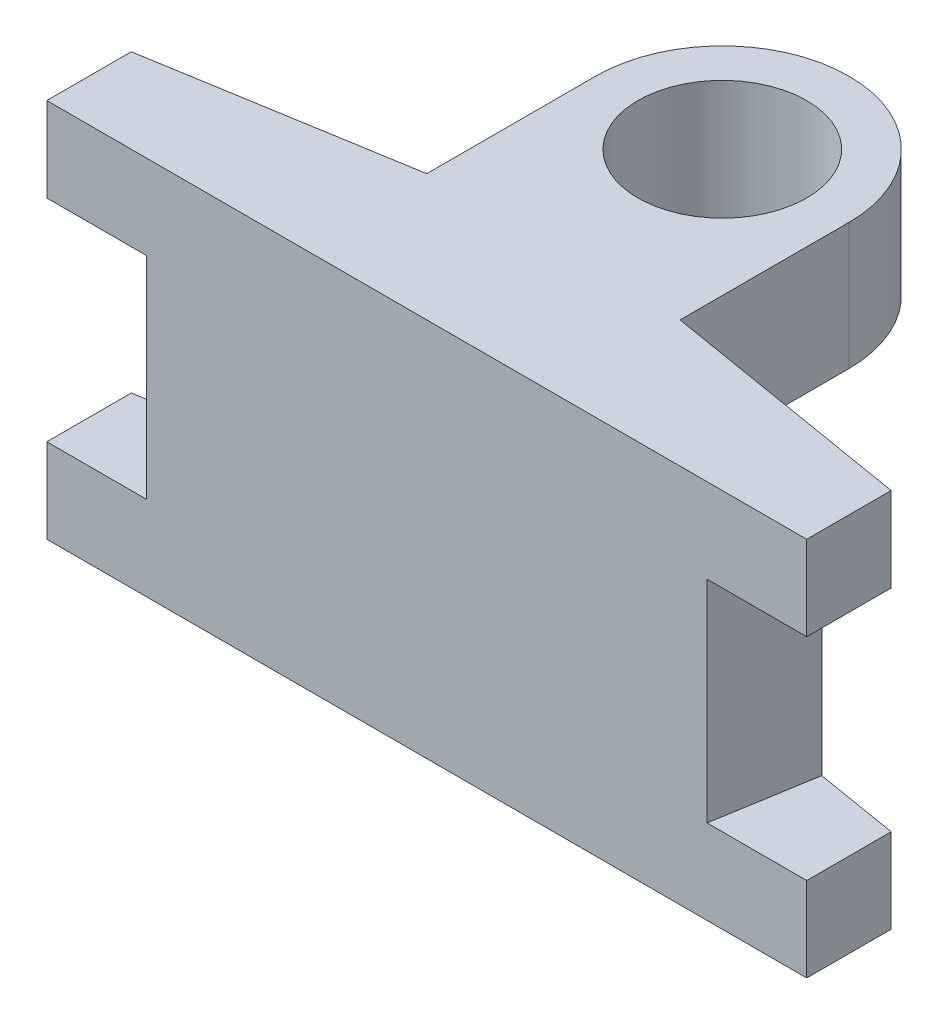
ISO-10303-21;
HEADER;
FILE_DESCRIPTION(('STEP AP214'),'2;1');
FILE_NAME('part.step','',(''),(''),'','','');
FILE_SCHEMA(('AUTOMOTIVE_DESIGN { 1 0 10303 214 1 1 1 1 }'));
ENDSEC;
DATA;
#1=APPLICATION_CONTEXT('core data for automotive mechanical design processes');
#2=APPLICATION_PROTOCOL_DEFINITION('international standard','automotive_design',2000,#1);
#3=PRODUCT_CONTEXT('',#1,'mechanical');
#4=PRODUCT('Part','Part','',(#3));
#5=PRODUCT_RELATED_PRODUCT_CATEGORY('part','',(#4));
#6=PRODUCT_DEFINITION_FORMATION('','',#4);
#7=PRODUCT_DEFINITION_CONTEXT('part definition',#1,'design');
#8=PRODUCT_DEFINITION('design','',#6,#7);
#9=PRODUCT_DEFINITION_SHAPE('','',#8);
#10=(LENGTH_UNIT() NAMED_UNIT(*) SI_UNIT(.MILLI.,.METRE.));
#11=(NAMED_UNIT(*) PLANE_ANGLE_UNIT() SI_UNIT($,.RADIAN.));
#12=(NAMED_UNIT(*) SI_UNIT($,.STERADIAN.) SOLID_ANGLE_UNIT());
#13=UNCERTAINTY_MEASURE_WITH_UNIT(LENGTH_MEASURE(1.E-05),#10,'distance_accuracy_value','');
#14=(GEOMETRIC_REPRESENTATION_CONTEXT(3) GLOBAL_UNCERTAINTY_ASSIGNED_CONTEXT((#13)) GLOBAL_UNIT_ASSIGNED_CONTEXT((#10,
#11,#12)) REPRESENTATION_CONTEXT('',''));
#15=CARTESIAN_POINT('',(0.,0.,0.));
#16=DIRECTION('',(0.,0.,1.));
#17=DIRECTION('',(1.,0.,0.));
#18=AXIS2_PLACEMENT_3D('',#15,#16,#17);
#19=CARTESIAN_POINT('',(0.,0.,20.));
#20=DIRECTION('',(0.,0.,1.));
#21=DIRECTION('',(1.,0.,0.));
#22=AXIS2_PLACEMENT_3D('',#19,#20,#21);
#23=PLANE('',#22);
#24=DIRECTION('',(0.,-1.,0.));
#25=VECTOR('',#24,1.);
#26=CARTESIAN_POINT('',(-33.1921504113325,0.,20.));
#27=LINE('',#26,#25);
#28=CARTESIAN_POINT('',(-33.1921504113325,12.5,20.));
#29=VERTEX_POINT('',#28);
#30=CARTESIAN_POINT('',(-33.1921504113325,-12.5,20.));
#31=VERTEX_POINT('',#30);
#32=EDGE_CURVE('E396',#29,#31,#27,.T.);
#33=ORIENTED_EDGE('',*,*,#32,.T.);
#34=DIRECTION('',(-1.,0.,0.));
#35=VECTOR('',#34,1.);
#36=CARTESIAN_POINT('',(-35.,-12.5,20.));
#37=LINE('',#36,#35);
#38=CARTESIAN_POINT('',(-45.,-12.5,20.));
#39=VERTEX_POINT('',#38);
#40=EDGE_CURVE('E211',#31,#39,#37,.T.);
#41=ORIENTED_EDGE('',*,*,#40,.T.);
#42=DIRECTION('',(0.,-1.,0.));
#43=VECTOR('',#42,1.);
#44=CARTESIAN_POINT('',(-45.,22.5,20.));
#45=LINE('',#44,#43);
#46=CARTESIAN_POINT('',(-45.,-22.5,20.));
#47=VERTEX_POINT('',#46);
#48=EDGE_CURVE('E227',#39,#47,#45,.T.);
#49=ORIENTED_EDGE('',*,*,#48,.T.);
#50=DIRECTION('',(1.,0.,0.));
#51=VECTOR('',#50,1.);
#52=CARTESIAN_POINT('',(15.,-22.5,20.));
#53=LINE('',#52,#51);
#54=CARTESIAN_POINT('',(45.,-22.5,20.));
#55=VERTEX_POINT('',#54);
#56=EDGE_CURVE('E316',#47,#55,#53,.T.);
#57=ORIENTED_EDGE('',*,*,#56,.T.);
#58=DIRECTION('',(0.,-1.,0.));
#59=VECTOR('',#58,1.);
#60=CARTESIAN_POINT('',(45.,22.5,20.));
#61=LINE('',#60,#59);
#62=CARTESIAN_POINT('',(45.,-12.5,20.));
#63=VERTEX_POINT('',#62);
#64=EDGE_CURVE('E268',#63,#55,#61,.T.);
#65=ORIENTED_EDGE('',*,*,#64,.F.);
#66=DIRECTION('',(1.,0.,0.));
#67=VECTOR('',#66,1.);
#68=CARTESIAN_POINT('',(35.,-12.5,20.));
#69=LINE('',#68,#67);
#70=CARTESIAN_POINT('',(33.1921504113325,-12.5,20.));
#71=VERTEX_POINT('',#70);
#72=EDGE_CURVE('E250',#71,#63,#69,.T.);
#73=ORIENTED_EDGE('',*,*,#72,.F.);
#74=DIRECTION('',(0.,-1.,0.));
#75=VECTOR('',#74,1.);
#76=CARTESIAN_POINT('',(33.1921504113325,0.,20.));
#77=LINE('',#76,#75);
#78=CARTESIAN_POINT('',(33.1921504113325,12.5,20.));
#79=VERTEX_POINT('',#78);
#80=EDGE_CURVE('E240',#79,#71,#77,.T.);
#81=ORIENTED_EDGE('',*,*,#80,.F.);
#82=DIRECTION('',(1.,0.,0.));
#83=VECTOR('',#82,1.);
#84=CARTESIAN_POINT('',(35.,12.5,20.));
#85=LINE('',#84,#83);
#86=CARTESIAN_POINT('',(45.,12.5,20.));
#87=VERTEX_POINT('',#86);
#88=EDGE_CURVE('E246',#79,#87,#85,.T.);
#89=ORIENTED_EDGE('',*,*,#88,.T.);
#90=CARTESIAN_POINT('',(45.,22.5,20.));
#91=VERTEX_POINT('',#90);
#92=EDGE_CURVE('E262',#91,#87,#61,.T.);
#93=ORIENTED_EDGE('',*,*,#92,.F.);
#94=DIRECTION('',(-1.,0.,0.));
#95=VECTOR('',#94,1.);
#96=CARTESIAN_POINT('',(15.,22.5,20.));
#97=LINE('',#96,#95);
#98=CARTESIAN_POINT('',(-45.,22.5,20.));
#99=VERTEX_POINT('',#98);
#100=EDGE_CURVE('E317',#91,#99,#97,.T.);
#101=ORIENTED_EDGE('',*,*,#100,.T.);
#102=CARTESIAN_POINT('',(-45.,12.5,20.));
#103=VERTEX_POINT('',#102);
#104=EDGE_CURVE('E225',#99,#103,#45,.T.);
#105=ORIENTED_EDGE('',*,*,#104,.T.);
#106=DIRECTION('',(-1.,0.,0.));
#107=VECTOR('',#106,1.);
#108=CARTESIAN_POINT('',(-35.,12.5,20.));
#109=LINE('',#108,#107);
#110=EDGE_CURVE('E54',#29,#103,#109,.T.);
#111=ORIENTED_EDGE('',*,*,#110,.F.);
#112=EDGE_LOOP('',(#33,#41,#49,#57,#65,#73,#81,#89,#93,#101,#105,#111));
#113=FACE_BOUND('',#112,.T.);
#114=ADVANCED_FACE('F39',(#113),#23,.T.);
#115=CARTESIAN_POINT('',(-45.,22.5,10.));
#116=DIRECTION('',(0.164398987305357,0.,0.986393923832144));
#117=DIRECTION('',(0.986393923832144,0.,-0.164398987305357));
#118=AXIS2_PLACEMENT_3D('',#115,#116,#117);
#119=PLANE('',#118);
#120=DIRECTION('',(0.986393923832144,0.,-0.164398987305358));
#121=VECTOR('',#120,1.);
#122=CARTESIAN_POINT('',(-45.,-12.5,10.));
#123=LINE('',#122,#121);
#124=CARTESIAN_POINT('',(-45.,-12.5,10.));
#125=VERTEX_POINT('',#124);
#126=CARTESIAN_POINT('',(-35.1329031029181,-12.5,8.35548385048635));
#127=VERTEX_POINT('',#126);
#128=EDGE_CURVE('E401',#125,#127,#123,.T.);
#129=ORIENTED_EDGE('',*,*,#128,.T.);
#130=DIRECTION('',(0.,1.,0.));
#131=VECTOR('',#130,1.);
#132=CARTESIAN_POINT('',(-35.1329031029181,-12.5,8.35548385048635));
#133=LINE('',#132,#131);
#134=CARTESIAN_POINT('',(-35.1329031029181,12.5,8.35548385048635));
#135=VERTEX_POINT('',#134);
#136=EDGE_CURVE('E204',#127,#135,#133,.T.);
#137=ORIENTED_EDGE('',*,*,#136,.T.);
#138=DIRECTION('',(-0.986393923832144,0.,0.164398987305357));
#139=VECTOR('',#138,1.);
#140=CARTESIAN_POINT('',(-35.1329031029181,12.5,8.35548385048635));
#141=LINE('',#140,#139);
#142=CARTESIAN_POINT('',(-45.,12.5,10.));
#143=VERTEX_POINT('',#142);
#144=EDGE_CURVE('E197',#135,#143,#141,.T.);
#145=ORIENTED_EDGE('',*,*,#144,.T.);
#146=DIRECTION('',(0.,-1.,0.));
#147=VECTOR('',#146,1.);
#148=CARTESIAN_POINT('',(-45.,22.5,10.));
#149=LINE('',#148,#147);
#150=CARTESIAN_POINT('',(-45.,22.5,10.));
#151=VERTEX_POINT('',#150);
#152=EDGE_CURVE('E203',#151,#143,#149,.T.);
#153=ORIENTED_EDGE('',*,*,#152,.F.);
#154=DIRECTION('',(-0.986393923832144,0.,0.164398987305357));
#155=VECTOR('',#154,1.);
#156=CARTESIAN_POINT('',(-45.,22.5,10.));
#157=LINE('',#156,#155);
#158=CARTESIAN_POINT('',(-15.,22.5,5.));
#159=VERTEX_POINT('',#158);
#160=EDGE_CURVE('E382',#159,#151,#157,.T.);
#161=ORIENTED_EDGE('',*,*,#160,.F.);
#162=DIRECTION('',(0.,-1.,0.));
#163=VECTOR('',#162,1.);
#164=CARTESIAN_POINT('',(-15.,22.5,5.));
#165=LINE('',#164,#163);
#166=CARTESIAN_POINT('',(-15.,-22.5,5.));
#167=VERTEX_POINT('',#166);
#168=EDGE_CURVE('E220',#159,#167,#165,.T.);
#169=ORIENTED_EDGE('',*,*,#168,.T.);
#170=DIRECTION('',(-0.986393923832144,0.,0.164398987305357));
#171=VECTOR('',#170,1.);
#172=CARTESIAN_POINT('',(-45.,-22.5,10.));
#173=LINE('',#172,#171);
#174=CARTESIAN_POINT('',(-45.,-22.5,10.));
#175=VERTEX_POINT('',#174);
#176=EDGE_CURVE('E381',#167,#175,#173,.T.);
#177=ORIENTED_EDGE('',*,*,#176,.T.);
#178=EDGE_CURVE('E217',#125,#175,#149,.T.);
#179=ORIENTED_EDGE('',*,*,#178,.F.);
#180=EDGE_LOOP('',(#129,#137,#145,#153,#161,#169,#177,#179));
#181=FACE_BOUND('',#180,.T.);
#182=ADVANCED_FACE('F200',(#181),#119,.F.);
#183=CARTESIAN_POINT('',(-45.,22.5,20.));
#184=DIRECTION('',(1.,0.,0.));
#185=DIRECTION('',(0.,0.,-1.));
#186=AXIS2_PLACEMENT_3D('',#183,#184,#185);
#187=PLANE('',#186);
#188=DIRECTION('',(0.,0.,-1.));
#189=VECTOR('',#188,1.);
#190=CARTESIAN_POINT('',(-45.,-12.5,20.));
#191=LINE('',#190,#189);
#192=EDGE_CURVE('E215',#39,#125,#191,.T.);
#193=ORIENTED_EDGE('',*,*,#192,.T.);
#194=ORIENTED_EDGE('',*,*,#178,.T.);
#195=DIRECTION('',(0.,0.,1.));
#196=VECTOR('',#195,1.);
#197=CARTESIAN_POINT('',(-45.,-22.5,20.));
#198=LINE('',#197,#196);
#199=EDGE_CURVE('E389',#175,#47,#198,.T.);
#200=ORIENTED_EDGE('',*,*,#199,.T.);
#201=ORIENTED_EDGE('',*,*,#48,.F.);
#202=EDGE_LOOP('',(#193,#194,#200,#201));
#203=FACE_BOUND('',#202,.T.);
#204=ADVANCED_FACE('F411',(#203),#187,.F.);
#205=DIRECTION('',(0.,0.,1.));
#206=VECTOR('',#205,1.);
#207=CARTESIAN_POINT('',(-45.,12.5,20.));
#208=LINE('',#207,#206);
#209=EDGE_CURVE('E206',#143,#103,#208,.T.);
#210=ORIENTED_EDGE('',*,*,#209,.T.);
#211=ORIENTED_EDGE('',*,*,#104,.F.);
#212=DIRECTION('',(0.,0.,1.));
#213=VECTOR('',#212,1.);
#214=CARTESIAN_POINT('',(-45.,22.5,20.));
#215=LINE('',#214,#213);
#216=EDGE_CURVE('E216',#151,#99,#215,.T.);
#217=ORIENTED_EDGE('',*,*,#216,.F.);
#218=ORIENTED_EDGE('',*,*,#152,.T.);
#219=EDGE_LOOP('',(#210,#211,#217,#218));
#220=FACE_BOUND('',#219,.T.);
#221=ADVANCED_FACE('F212',(#220),#187,.F.);
#222=CARTESIAN_POINT('',(-15.,-22.5,20.));
#223=DIRECTION('',(1.,0.,0.));
#224=DIRECTION('',(0.,0.,-1.));
#225=AXIS2_PLACEMENT_3D('',#222,#223,#224);
#226=PLANE('',#225);
#227=ORIENTED_EDGE('',*,*,#168,.F.);
#228=DIRECTION('',(0.,0.,-1.));
#229=VECTOR('',#228,1.);
#230=CARTESIAN_POINT('',(-15.,22.5,20.));
#231=LINE('',#230,#229);
#232=CARTESIAN_POINT('',(-15.,22.5,-15.));
#233=VERTEX_POINT('',#232);
#234=EDGE_CURVE('E325',#159,#233,#231,.T.);
#235=ORIENTED_EDGE('',*,*,#234,.T.);
#236=DIRECTION('',(0.,1.,0.));
#237=VECTOR('',#236,1.);
#238=CARTESIAN_POINT('',(-15.,7.50000000000001,-15.));
#239=LINE('',#238,#237);
#240=CARTESIAN_POINT('',(-15.,7.50000000000001,-15.));
#241=VERTEX_POINT('',#240);
#242=EDGE_CURVE('E345',#233,#241,#239,.F.);
#243=ORIENTED_EDGE('',*,*,#242,.T.);
#244=DIRECTION('',(0.,0.,1.));
#245=VECTOR('',#244,1.);
#246=CARTESIAN_POINT('',(-15.,7.50000000000001,-30.));
#247=LINE('',#246,#245);
#248=CARTESIAN_POINT('',(-15.,7.50000000000001,0.));
#249=VERTEX_POINT('',#248);
#250=EDGE_CURVE('E283',#241,#249,#247,.T.);
#251=ORIENTED_EDGE('',*,*,#250,.T.);
#252=DIRECTION('',(0.,-1.,0.));
#253=VECTOR('',#252,1.);
#254=CARTESIAN_POINT('',(-15.,-22.5,0.));
#255=LINE('',#254,#253);
#256=CARTESIAN_POINT('',(-15.,-22.5,0.));
#257=VERTEX_POINT('',#256);
#258=EDGE_CURVE('E306',#249,#257,#255,.T.);
#259=ORIENTED_EDGE('',*,*,#258,.T.);
#260=DIRECTION('',(0.,0.,-1.));
#261=VECTOR('',#260,1.);
#262=CARTESIAN_POINT('',(-15.,-22.5,20.));
#263=LINE('',#262,#261);
#264=EDGE_CURVE('E337',#167,#257,#263,.T.);
#265=ORIENTED_EDGE('',*,*,#264,.F.);
#266=EDGE_LOOP('',(#227,#235,#243,#251,#259,#265));
#267=FACE_BOUND('',#266,.T.);
#268=ADVANCED_FACE('F380',(#267),#226,.F.);
#269=CARTESIAN_POINT('',(45.,22.5,20.));
#270=DIRECTION('',(1.,0.,0.));
#271=DIRECTION('',(0.,0.,-1.));
#272=AXIS2_PLACEMENT_3D('',#269,#270,#271);
#273=PLANE('',#272);
#274=DIRECTION('',(0.,0.,-1.));
#275=VECTOR('',#274,1.);
#276=CARTESIAN_POINT('',(45.,-12.5,20.));
#277=LINE('',#276,#275);
#278=CARTESIAN_POINT('',(45.,-12.5,10.));
#279=VERTEX_POINT('',#278);
#280=EDGE_CURVE('E242',#63,#279,#277,.T.);
#281=ORIENTED_EDGE('',*,*,#280,.F.);
#282=ORIENTED_EDGE('',*,*,#64,.T.);
#283=DIRECTION('',(0.,0.,1.));
#284=VECTOR('',#283,1.);
#285=CARTESIAN_POINT('',(45.,-22.5,20.));
#286=LINE('',#285,#284);
#287=CARTESIAN_POINT('',(45.,-22.5,10.));
#288=VERTEX_POINT('',#287);
#289=EDGE_CURVE('E258',#288,#55,#286,.T.);
#290=ORIENTED_EDGE('',*,*,#289,.F.);
#291=DIRECTION('',(0.,-1.,0.));
#292=VECTOR('',#291,1.);
#293=CARTESIAN_POINT('',(45.,22.5,10.));
#294=LINE('',#293,#292);
#295=EDGE_CURVE('E275',#279,#288,#294,.T.);
#296=ORIENTED_EDGE('',*,*,#295,.F.);
#297=EDGE_LOOP('',(#281,#282,#290,#296));
#298=FACE_BOUND('',#297,.T.);
#299=ADVANCED_FACE('F419',(#298),#273,.T.);
#300=CARTESIAN_POINT('',(0.,0.,0.));
#301=DIRECTION('',(0.,0.,1.));
#302=DIRECTION('',(1.,0.,0.));
#303=AXIS2_PLACEMENT_3D('',#300,#301,#302);
#304=PLANE('',#303);
#305=DIRECTION('',(-1.,0.,0.));
#306=VECTOR('',#305,1.);
#307=CARTESIAN_POINT('',(15.,7.50000000000001,0.));
#308=LINE('',#307,#306);
#309=CARTESIAN_POINT('',(15.,7.5,0.));
#310=VERTEX_POINT('',#309);
#311=EDGE_CURVE('E278',#310,#249,#308,.T.);
#312=ORIENTED_EDGE('',*,*,#311,.F.);
#313=DIRECTION('',(0.,1.,0.));
#314=VECTOR('',#313,1.);
#315=CARTESIAN_POINT('',(15.,-22.5,0.));
#316=LINE('',#315,#314);
#317=CARTESIAN_POINT('',(15.,-22.5,0.));
#318=VERTEX_POINT('',#317);
#319=EDGE_CURVE('E319',#318,#310,#316,.T.);
#320=ORIENTED_EDGE('',*,*,#319,.F.);
#321=DIRECTION('',(1.,0.,0.));
#322=VECTOR('',#321,1.);
#323=CARTESIAN_POINT('',(15.,-22.5,0.));
#324=LINE('',#323,#322);
#325=CARTESIAN_POINT('',(9.99999999999999,-22.5,0.));
#326=VERTEX_POINT('',#325);
#327=EDGE_CURVE('E324',#326,#318,#324,.T.);
#328=ORIENTED_EDGE('',*,*,#327,.F.);
#329=DIRECTION('',(0.,-1.,0.));
#330=VECTOR('',#329,1.);
#331=CARTESIAN_POINT('',(10.,-7.5,0.));
#332=LINE('',#331,#330);
#333=CARTESIAN_POINT('',(10.,-7.5,0.));
#334=VERTEX_POINT('',#333);
#335=EDGE_CURVE('E301',#334,#326,#332,.T.);
#336=ORIENTED_EDGE('',*,*,#335,.F.);
#337=CARTESIAN_POINT('',(0.,-7.49999999999999,0.));
#338=DIRECTION('',(0.,0.,-1.));
#339=DIRECTION('',(-1.,0.,0.));
#340=AXIS2_PLACEMENT_3D('',#337,#338,#339);
#341=CIRCLE('',#340,10.);
#342=CARTESIAN_POINT('',(-10.,-7.49999999999999,0.));
#343=VERTEX_POINT('',#342);
#344=EDGE_CURVE('E286',#343,#334,#341,.T.);
#345=ORIENTED_EDGE('',*,*,#344,.F.);
#346=DIRECTION('',(0.,1.,0.));
#347=VECTOR('',#346,1.);
#348=CARTESIAN_POINT('',(-10.,-22.5,0.));
#349=LINE('',#348,#347);
#350=CARTESIAN_POINT('',(-10.,-22.5,0.));
#351=VERTEX_POINT('',#350);
#352=EDGE_CURVE('E295',#351,#343,#349,.T.);
#353=ORIENTED_EDGE('',*,*,#352,.F.);
#354=EDGE_CURVE('E326',#257,#351,#324,.T.);
#355=ORIENTED_EDGE('',*,*,#354,.F.);
#356=ORIENTED_EDGE('',*,*,#258,.F.);
#357=EDGE_LOOP('',(#312,#320,#328,#336,#345,#353,#355,#356));
#358=FACE_BOUND('',#357,.T.);
#359=ADVANCED_FACE('F367',(#358),#304,.F.);
#360=CARTESIAN_POINT('',(15.,-22.5,20.));
#361=DIRECTION('',(0.,1.,0.));
#362=DIRECTION('',(0.,0.,1.));
#363=AXIS2_PLACEMENT_3D('',#360,#361,#362);
#364=PLANE('',#363);
#365=ORIENTED_EDGE('',*,*,#354,.T.);
#366=DIRECTION('',(0.,0.,-1.));
#367=VECTOR('',#366,1.);
#368=CARTESIAN_POINT('',(-10.,-22.5,8.));
#369=LINE('',#368,#367);
#370=CARTESIAN_POINT('',(-10.,-22.5,8.));
#371=VERTEX_POINT('',#370);
#372=EDGE_CURVE('E310',#371,#351,#369,.T.);
#373=ORIENTED_EDGE('',*,*,#372,.F.);
#374=DIRECTION('',(-1.,0.,0.));
#375=VECTOR('',#374,1.);
#376=CARTESIAN_POINT('',(9.99999999999999,-22.5,8.));
#377=LINE('',#376,#375);
#378=CARTESIAN_POINT('',(9.99999999999999,-22.5,8.));
#379=VERTEX_POINT('',#378);
#380=EDGE_CURVE('E293',#379,#371,#377,.T.);
#381=ORIENTED_EDGE('',*,*,#380,.F.);
#382=DIRECTION('',(0.,0.,-1.));
#383=VECTOR('',#382,1.);
#384=CARTESIAN_POINT('',(9.99999999999999,-22.5,8.));
#385=LINE('',#384,#383);
#386=EDGE_CURVE('E313',#379,#326,#385,.T.);
#387=ORIENTED_EDGE('',*,*,#386,.T.);
#388=ORIENTED_EDGE('',*,*,#327,.T.);
#389=DIRECTION('',(0.,0.,-1.));
#390=VECTOR('',#389,1.);
#391=CARTESIAN_POINT('',(15.,-22.5,20.));
#392=LINE('',#391,#390);
#393=CARTESIAN_POINT('',(15.,-22.5,5.));
#394=VERTEX_POINT('',#393);
#395=EDGE_CURVE('E331',#394,#318,#392,.T.);
#396=ORIENTED_EDGE('',*,*,#395,.F.);
#397=DIRECTION('',(0.986393923832144,0.,0.164398987305357));
#398=VECTOR('',#397,1.);
#399=CARTESIAN_POINT('',(45.,-22.5,10.));
#400=LINE('',#399,#398);
#401=EDGE_CURVE('E247',#394,#288,#400,.T.);
#402=ORIENTED_EDGE('',*,*,#401,.T.);
#403=ORIENTED_EDGE('',*,*,#289,.T.);
#404=ORIENTED_EDGE('',*,*,#56,.F.);
#405=ORIENTED_EDGE('',*,*,#199,.F.);
#406=ORIENTED_EDGE('',*,*,#176,.F.);
#407=ORIENTED_EDGE('',*,*,#264,.T.);
#408=EDGE_LOOP('',(#365,#373,#381,#387,#388,#396,#402,#403,#404,#405,#406,#407));
#409=FACE_BOUND('',#408,.T.);
#410=ADVANCED_FACE('F384',(#409),#364,.F.);
#411=CARTESIAN_POINT('',(15.,-22.5,20.));
#412=DIRECTION('',(-1.,0.,0.));
#413=DIRECTION('',(0.,0.,1.));
#414=AXIS2_PLACEMENT_3D('',#411,#412,#413);
#415=PLANE('',#414);
#416=DIRECTION('',(0.,0.,-1.));
#417=VECTOR('',#416,1.);
#418=CARTESIAN_POINT('',(15.,22.5,20.));
#419=LINE('',#418,#417);
#420=CARTESIAN_POINT('',(15.,22.5,5.));
#421=VERTEX_POINT('',#420);
#422=CARTESIAN_POINT('',(15.,22.5,-15.));
#423=VERTEX_POINT('',#422);
#424=EDGE_CURVE('E335',#421,#423,#419,.T.);
#425=ORIENTED_EDGE('',*,*,#424,.F.);
#426=DIRECTION('',(0.,-1.,0.));
#427=VECTOR('',#426,1.);
#428=CARTESIAN_POINT('',(15.,22.5,5.));
#429=LINE('',#428,#427);
#430=EDGE_CURVE('E259',#421,#394,#429,.T.);
#431=ORIENTED_EDGE('',*,*,#430,.T.);
#432=ORIENTED_EDGE('',*,*,#395,.T.);
#433=ORIENTED_EDGE('',*,*,#319,.T.);
#434=DIRECTION('',(0.,0.,1.));
#435=VECTOR('',#434,1.);
#436=CARTESIAN_POINT('',(15.,7.50000000000001,-30.));
#437=LINE('',#436,#435);
#438=CARTESIAN_POINT('',(15.,7.50000000000001,-15.));
#439=VERTEX_POINT('',#438);
#440=EDGE_CURVE('E281',#439,#310,#437,.T.);
#441=ORIENTED_EDGE('',*,*,#440,.F.);
#442=DIRECTION('',(0.,-1.,0.));
#443=VECTOR('',#442,1.);
#444=CARTESIAN_POINT('',(15.,22.5,-15.));
#445=LINE('',#444,#443);
#446=EDGE_CURVE('E11',#439,#423,#445,.F.);
#447=ORIENTED_EDGE('',*,*,#446,.T.);
#448=EDGE_LOOP('',(#425,#431,#432,#433,#441,#447));
#449=FACE_BOUND('',#448,.T.);
#450=ADVANCED_FACE('F364',(#449),#415,.F.);
#451=CARTESIAN_POINT('',(15.,22.5,20.));
#452=DIRECTION('',(0.,-1.,0.));
#453=DIRECTION('',(0.,0.,-1.));
#454=AXIS2_PLACEMENT_3D('',#451,#452,#453);
#455=PLANE('',#454);
#456=CARTESIAN_POINT('',(0.,22.5,-15.));
#457=DIRECTION('',(0.,-1.,0.));
#458=DIRECTION('',(0.,0.,-1.));
#459=AXIS2_PLACEMENT_3D('',#456,#457,#458);
#460=CIRCLE('',#459,10.);
#461=CARTESIAN_POINT('',(0.,22.5,-25.));
#462=VERTEX_POINT('',#461);
#463=EDGE_CURVE('E280',#462,#462,#460,.T.);
#464=ORIENTED_EDGE('',*,*,#463,.T.);
#465=EDGE_LOOP('',(#464));
#466=FACE_BOUND('',#465,.T.);
#467=CARTESIAN_POINT('',(0.,22.5,-15.));
#468=DIRECTION('',(0.,-1.,0.));
#469=DIRECTION('',(0.,0.,-1.));
#470=AXIS2_PLACEMENT_3D('',#467,#468,#469);
#471=CIRCLE('',#470,15.);
#472=CARTESIAN_POINT('',(0.,22.5,-30.));
#473=VERTEX_POINT('',#472);
#474=EDGE_CURVE('E338',#423,#473,#471,.F.);
#475=ORIENTED_EDGE('',*,*,#474,.T.);
#476=CARTESIAN_POINT('',(0.,22.5,-15.));
#477=DIRECTION('',(0.,-1.,0.));
#478=DIRECTION('',(0.,0.,-1.));
#479=AXIS2_PLACEMENT_3D('',#476,#477,#478);
#480=CIRCLE('',#479,15.);
#481=EDGE_CURVE('E336',#473,#233,#480,.F.);
#482=ORIENTED_EDGE('',*,*,#481,.T.);
#483=ORIENTED_EDGE('',*,*,#234,.F.);
#484=ORIENTED_EDGE('',*,*,#160,.T.);
#485=ORIENTED_EDGE('',*,*,#216,.T.);
#486=ORIENTED_EDGE('',*,*,#100,.F.);
#487=DIRECTION('',(0.,0.,1.));
#488=VECTOR('',#487,1.);
#489=CARTESIAN_POINT('',(45.,22.5,20.));
#490=LINE('',#489,#488);
#491=CARTESIAN_POINT('',(45.,22.5,10.));
#492=VERTEX_POINT('',#491);
#493=EDGE_CURVE('E254',#492,#91,#490,.T.);
#494=ORIENTED_EDGE('',*,*,#493,.F.);
#495=DIRECTION('',(0.986393923832144,0.,0.164398987305357));
#496=VECTOR('',#495,1.);
#497=CARTESIAN_POINT('',(45.,22.5,10.));
#498=LINE('',#497,#496);
#499=EDGE_CURVE('E252',#421,#492,#498,.T.);
#500=ORIENTED_EDGE('',*,*,#499,.F.);
#501=ORIENTED_EDGE('',*,*,#424,.T.);
#502=EDGE_LOOP('',(#475,#482,#483,#484,#485,#486,#494,#500,#501));
#503=FACE_BOUND('',#502,.T.);
#504=ADVANCED_FACE('F357',(#466,#503),#455,.F.);
#505=CARTESIAN_POINT('',(0.,-7.49999999999999,8.));
#506=DIRECTION('',(0.,0.,-1.));
#507=DIRECTION('',(-1.,0.,0.));
#508=AXIS2_PLACEMENT_3D('',#505,#506,#507);
#509=CYLINDRICAL_SURFACE('',#508,10.);
#510=ORIENTED_EDGE('',*,*,#344,.T.);
#511=DIRECTION('',(0.,0.,-1.));
#512=VECTOR('',#511,1.);
#513=CARTESIAN_POINT('',(10.,-7.5,8.));
#514=LINE('',#513,#512);
#515=CARTESIAN_POINT('',(10.,-7.5,8.));
#516=VERTEX_POINT('',#515);
#517=EDGE_CURVE('E296',#516,#334,#514,.T.);
#518=ORIENTED_EDGE('',*,*,#517,.F.);
#519=CARTESIAN_POINT('',(0.,-7.49999999999999,8.));
#520=DIRECTION('',(0.,0.,-1.));
#521=DIRECTION('',(-1.,0.,0.));
#522=AXIS2_PLACEMENT_3D('',#519,#520,#521);
#523=CIRCLE('',#522,10.);
#524=CARTESIAN_POINT('',(-10.,-7.49999999999999,8.));
#525=VERTEX_POINT('',#524);
#526=EDGE_CURVE('E290',#525,#516,#523,.T.);
#527=ORIENTED_EDGE('',*,*,#526,.F.);
#528=DIRECTION('',(0.,0.,-1.));
#529=VECTOR('',#528,1.);
#530=CARTESIAN_POINT('',(-10.,-7.49999999999999,8.));
#531=LINE('',#530,#529);
#532=EDGE_CURVE('E308',#525,#343,#531,.T.);
#533=ORIENTED_EDGE('',*,*,#532,.T.);
#534=EDGE_LOOP('',(#510,#518,#527,#533));
#535=FACE_BOUND('',#534,.T.);
#536=ADVANCED_FACE('F457',(#535),#509,.F.);
#537=CARTESIAN_POINT('',(-10.,-22.5,8.));
#538=DIRECTION('',(-1.,0.,0.));
#539=DIRECTION('',(0.,-1.,0.));
#540=AXIS2_PLACEMENT_3D('',#537,#538,#539);
#541=PLANE('',#540);
#542=ORIENTED_EDGE('',*,*,#352,.T.);
#543=ORIENTED_EDGE('',*,*,#532,.F.);
#544=DIRECTION('',(0.,1.,0.));
#545=VECTOR('',#544,1.);
#546=CARTESIAN_POINT('',(-10.,-22.5,8.));
#547=LINE('',#546,#545);
#548=EDGE_CURVE('E300',#371,#525,#547,.T.);
#549=ORIENTED_EDGE('',*,*,#548,.F.);
#550=ORIENTED_EDGE('',*,*,#372,.T.);
#551=EDGE_LOOP('',(#542,#543,#549,#550));
#552=FACE_BOUND('',#551,.T.);
#553=ADVANCED_FACE('F491',(#552),#541,.F.);
#554=CARTESIAN_POINT('',(10.,-7.5,8.));
#555=DIRECTION('',(1.,0.,0.));
#556=DIRECTION('',(0.,1.,0.));
#557=AXIS2_PLACEMENT_3D('',#554,#555,#556);
#558=PLANE('',#557);
#559=ORIENTED_EDGE('',*,*,#335,.T.);
#560=ORIENTED_EDGE('',*,*,#386,.F.);
#561=DIRECTION('',(0.,-1.,0.));
#562=VECTOR('',#561,1.);
#563=CARTESIAN_POINT('',(10.,-7.5,8.));
#564=LINE('',#563,#562);
#565=EDGE_CURVE('E292',#516,#379,#564,.T.);
#566=ORIENTED_EDGE('',*,*,#565,.F.);
#567=ORIENTED_EDGE('',*,*,#517,.T.);
#568=EDGE_LOOP('',(#559,#560,#566,#567));
#569=FACE_BOUND('',#568,.T.);
#570=ADVANCED_FACE('F484',(#569),#558,.F.);
#571=CARTESIAN_POINT('',(0.,-7.49999999999999,8.));
#572=DIRECTION('',(0.,0.,-1.));
#573=DIRECTION('',(-1.,0.,0.));
#574=AXIS2_PLACEMENT_3D('',#571,#572,#573);
#575=PLANE('',#574);
#576=ORIENTED_EDGE('',*,*,#526,.T.);
#577=ORIENTED_EDGE('',*,*,#565,.T.);
#578=ORIENTED_EDGE('',*,*,#380,.T.);
#579=ORIENTED_EDGE('',*,*,#548,.T.);
#580=EDGE_LOOP('',(#576,#577,#578,#579));
#581=FACE_BOUND('',#580,.T.);
#582=ADVANCED_FACE('F479',(#581),#575,.T.);
#583=CARTESIAN_POINT('',(15.,7.50000000000001,-30.));
#584=DIRECTION('',(0.,1.,0.));
#585=DIRECTION('',(0.,0.,1.));
#586=AXIS2_PLACEMENT_3D('',#583,#584,#585);
#587=PLANE('',#586);
#588=CARTESIAN_POINT('',(0.,7.50000000000001,-15.));
#589=DIRECTION('',(0.,-1.,0.));
#590=DIRECTION('',(0.,0.,-1.));
#591=AXIS2_PLACEMENT_3D('',#588,#589,#590);
#592=CIRCLE('',#591,10.);
#593=CARTESIAN_POINT('',(0.,7.50000000000001,-25.));
#594=VERTEX_POINT('',#593);
#595=EDGE_CURVE('E270',#594,#594,#592,.T.);
#596=ORIENTED_EDGE('',*,*,#595,.F.);
#597=EDGE_LOOP('',(#596));
#598=FACE_BOUND('',#597,.T.);
#599=ORIENTED_EDGE('',*,*,#250,.F.);
#600=CARTESIAN_POINT('',(0.,7.50000000000001,-15.));
#601=DIRECTION('',(0.,1.,0.));
#602=DIRECTION('',(0.,0.,1.));
#603=AXIS2_PLACEMENT_3D('',#600,#601,#602);
#604=CIRCLE('',#603,15.);
#605=CARTESIAN_POINT('',(0.,7.50000000000001,-30.));
#606=VERTEX_POINT('',#605);
#607=EDGE_CURVE('E48',#241,#606,#604,.F.);
#608=ORIENTED_EDGE('',*,*,#607,.T.);
#609=CARTESIAN_POINT('',(0.,7.50000000000001,-15.));
#610=DIRECTION('',(0.,1.,0.));
#611=DIRECTION('',(0.,0.,1.));
#612=AXIS2_PLACEMENT_3D('',#609,#610,#611);
#613=CIRCLE('',#612,15.);
#614=EDGE_CURVE('E63',#606,#439,#613,.F.);
#615=ORIENTED_EDGE('',*,*,#614,.T.);
#616=ORIENTED_EDGE('',*,*,#440,.T.);
#617=ORIENTED_EDGE('',*,*,#311,.T.);
#618=EDGE_LOOP('',(#599,#608,#615,#616,#617));
#619=FACE_BOUND('',#618,.T.);
#620=ADVANCED_FACE('F346',(#598,#619),#587,.F.);
#621=CARTESIAN_POINT('',(0.,0.,-15.));
#622=DIRECTION('',(0.,1.,0.));
#623=DIRECTION('',(0.,0.,1.));
#624=AXIS2_PLACEMENT_3D('',#621,#622,#623);
#625=CYLINDRICAL_SURFACE('',#624,15.);
#626=ORIENTED_EDGE('',*,*,#446,.F.);
#627=ORIENTED_EDGE('',*,*,#614,.F.);
#628=DIRECTION('',(0.,-1.,0.));
#629=VECTOR('',#628,1.);
#630=CARTESIAN_POINT('',(0.,7.50000000000001,-30.));
#631=LINE('',#630,#629);
#632=EDGE_CURVE('E43',#473,#606,#631,.T.);
#633=ORIENTED_EDGE('',*,*,#632,.F.);
#634=ORIENTED_EDGE('',*,*,#474,.F.);
#635=EDGE_LOOP('',(#626,#627,#633,#634));
#636=FACE_BOUND('',#635,.T.);
#637=ADVANCED_FACE('F41',(#636),#625,.T.);
#638=CARTESIAN_POINT('',(0.,0.,-15.));
#639=DIRECTION('',(0.,-1.,0.));
#640=DIRECTION('',(0.,0.,-1.));
#641=AXIS2_PLACEMENT_3D('',#638,#639,#640);
#642=CYLINDRICAL_SURFACE('',#641,15.);
#643=ORIENTED_EDGE('',*,*,#607,.F.);
#644=ORIENTED_EDGE('',*,*,#242,.F.);
#645=ORIENTED_EDGE('',*,*,#481,.F.);
#646=ORIENTED_EDGE('',*,*,#632,.T.);
#647=EDGE_LOOP('',(#643,#644,#645,#646));
#648=FACE_BOUND('',#647,.T.);
#649=ADVANCED_FACE('F356',(#648),#642,.T.);
#650=CARTESIAN_POINT('',(0.,37.5,-15.));
#651=DIRECTION('',(0.,-1.,0.));
#652=DIRECTION('',(0.,0.,-1.));
#653=AXIS2_PLACEMENT_3D('',#650,#651,#652);
#654=CYLINDRICAL_SURFACE('',#653,10.);
#655=ORIENTED_EDGE('',*,*,#595,.T.);
#656=EDGE_LOOP('',(#655));
#657=FACE_BOUND('',#656,.T.);
#658=ORIENTED_EDGE('',*,*,#463,.F.);
#659=EDGE_LOOP('',(#658));
#660=FACE_BOUND('',#659,.T.);
#661=ADVANCED_FACE('F468',(#657,#660),#654,.F.);
#662=DIRECTION('',(0.,0.,1.));
#663=VECTOR('',#662,1.);
#664=CARTESIAN_POINT('',(45.,12.5,20.));
#665=LINE('',#664,#663);
#666=CARTESIAN_POINT('',(45.,12.5,10.));
#667=VERTEX_POINT('',#666);
#668=EDGE_CURVE('E244',#667,#87,#665,.T.);
#669=ORIENTED_EDGE('',*,*,#668,.F.);
#670=EDGE_CURVE('E267',#492,#667,#294,.T.);
#671=ORIENTED_EDGE('',*,*,#670,.F.);
#672=ORIENTED_EDGE('',*,*,#493,.T.);
#673=ORIENTED_EDGE('',*,*,#92,.T.);
#674=EDGE_LOOP('',(#669,#671,#672,#673));
#675=FACE_BOUND('',#674,.T.);
#676=ADVANCED_FACE('F436',(#675),#273,.T.);
#677=CARTESIAN_POINT('',(45.,22.5,10.));
#678=DIRECTION('',(0.164398987305357,0.,-0.986393923832144));
#679=DIRECTION('',(-0.986393923832144,0.,-0.164398987305357));
#680=AXIS2_PLACEMENT_3D('',#677,#678,#679);
#681=PLANE('',#680);
#682=DIRECTION('',(0.986393923832144,0.,0.164398987305357));
#683=VECTOR('',#682,1.);
#684=CARTESIAN_POINT('',(35.1329031029181,12.5,8.35548385048635));
#685=LINE('',#684,#683);
#686=CARTESIAN_POINT('',(35.1329031029181,12.5,8.35548385048635));
#687=VERTEX_POINT('',#686);
#688=EDGE_CURVE('E231',#687,#667,#685,.T.);
#689=ORIENTED_EDGE('',*,*,#688,.F.);
#690=DIRECTION('',(0.,1.,0.));
#691=VECTOR('',#690,1.);
#692=CARTESIAN_POINT('',(35.1329031029181,-12.5,8.35548385048635));
#693=LINE('',#692,#691);
#694=CARTESIAN_POINT('',(35.1329031029181,-12.5,8.35548385048635));
#695=VERTEX_POINT('',#694);
#696=EDGE_CURVE('E229',#695,#687,#693,.T.);
#697=ORIENTED_EDGE('',*,*,#696,.F.);
#698=DIRECTION('',(-0.986393923832144,0.,-0.164398987305358));
#699=VECTOR('',#698,1.);
#700=CARTESIAN_POINT('',(45.,-12.5,10.));
#701=LINE('',#700,#699);
#702=EDGE_CURVE('E219',#279,#695,#701,.T.);
#703=ORIENTED_EDGE('',*,*,#702,.F.);
#704=ORIENTED_EDGE('',*,*,#295,.T.);
#705=ORIENTED_EDGE('',*,*,#401,.F.);
#706=ORIENTED_EDGE('',*,*,#430,.F.);
#707=ORIENTED_EDGE('',*,*,#499,.T.);
#708=ORIENTED_EDGE('',*,*,#670,.T.);
#709=EDGE_LOOP('',(#689,#697,#703,#704,#705,#706,#707,#708));
#710=FACE_BOUND('',#709,.T.);
#711=ADVANCED_FACE('F431',(#710),#681,.T.);
#712=CARTESIAN_POINT('',(35.,-12.5,20.));
#713=DIRECTION('',(0.,-1.,0.));
#714=DIRECTION('',(0.,0.,-1.));
#715=AXIS2_PLACEMENT_3D('',#712,#713,#714);
#716=PLANE('',#715);
#717=ORIENTED_EDGE('',*,*,#280,.T.);
#718=ORIENTED_EDGE('',*,*,#702,.T.);
#719=DIRECTION('',(0.164398987305357,0.,-0.986393923832144));
#720=VECTOR('',#719,1.);
#721=CARTESIAN_POINT('',(31.8896598596748,-12.5,27.8149433099458));
#722=LINE('',#721,#720);
#723=EDGE_CURVE('E233',#71,#695,#722,.T.);
#724=ORIENTED_EDGE('',*,*,#723,.F.);
#725=ORIENTED_EDGE('',*,*,#72,.T.);
#726=EDGE_LOOP('',(#717,#718,#724,#725));
#727=FACE_BOUND('',#726,.T.);
#728=ADVANCED_FACE('F430',(#727),#716,.F.);
#729=CARTESIAN_POINT('',(35.,12.5,20.));
#730=DIRECTION('',(0.,1.,0.));
#731=DIRECTION('',(0.,0.,1.));
#732=AXIS2_PLACEMENT_3D('',#729,#730,#731);
#733=PLANE('',#732);
#734=ORIENTED_EDGE('',*,*,#668,.T.);
#735=ORIENTED_EDGE('',*,*,#88,.F.);
#736=DIRECTION('',(0.164398987305357,0.,-0.986393923832144));
#737=VECTOR('',#736,1.);
#738=CARTESIAN_POINT('',(31.8896598596748,12.5,27.8149433099458));
#739=LINE('',#738,#737);
#740=EDGE_CURVE('E232',#79,#687,#739,.T.);
#741=ORIENTED_EDGE('',*,*,#740,.T.);
#742=ORIENTED_EDGE('',*,*,#688,.T.);
#743=EDGE_LOOP('',(#734,#735,#741,#742));
#744=FACE_BOUND('',#743,.T.);
#745=ADVANCED_FACE('F432',(#744),#733,.F.);
#746=CARTESIAN_POINT('',(31.8896598596748,-12.5,27.8149433099458));
#747=DIRECTION('',(-0.986393923832144,0.,-0.164398987305357));
#748=DIRECTION('',(-0.164398987305357,0.,0.986393923832144));
#749=AXIS2_PLACEMENT_3D('',#746,#747,#748);
#750=PLANE('',#749);
#751=ORIENTED_EDGE('',*,*,#80,.T.);
#752=ORIENTED_EDGE('',*,*,#723,.T.);
#753=ORIENTED_EDGE('',*,*,#696,.T.);
#754=ORIENTED_EDGE('',*,*,#740,.F.);
#755=EDGE_LOOP('',(#751,#752,#753,#754));
#756=FACE_BOUND('',#755,.T.);
#757=ADVANCED_FACE('F426',(#756),#750,.F.);
#758=CARTESIAN_POINT('',(-35.,-12.5,20.));
#759=DIRECTION('',(0.,1.,0.));
#760=DIRECTION('',(0.,0.,1.));
#761=AXIS2_PLACEMENT_3D('',#758,#759,#760);
#762=PLANE('',#761);
#763=ORIENTED_EDGE('',*,*,#128,.F.);
#764=ORIENTED_EDGE('',*,*,#192,.F.);
#765=ORIENTED_EDGE('',*,*,#40,.F.);
#766=DIRECTION('',(-0.164398987305357,0.,-0.986393923832144));
#767=VECTOR('',#766,1.);
#768=CARTESIAN_POINT('',(-31.078849048864,-12.5,32.6798081748107));
#769=LINE('',#768,#767);
#770=EDGE_CURVE('E397',#31,#127,#769,.T.);
#771=ORIENTED_EDGE('',*,*,#770,.T.);
#772=EDGE_LOOP('',(#763,#764,#765,#771));
#773=FACE_BOUND('',#772,.T.);
#774=ADVANCED_FACE('F408',(#773),#762,.T.);
#775=CARTESIAN_POINT('',(-35.,12.5,20.));
#776=DIRECTION('',(0.,-1.,0.));
#777=DIRECTION('',(0.,0.,-1.));
#778=AXIS2_PLACEMENT_3D('',#775,#776,#777);
#779=PLANE('',#778);
#780=ORIENTED_EDGE('',*,*,#209,.F.);
#781=ORIENTED_EDGE('',*,*,#144,.F.);
#782=DIRECTION('',(-0.164398987305357,0.,-0.986393923832144));
#783=VECTOR('',#782,1.);
#784=CARTESIAN_POINT('',(-31.078849048864,12.5,32.6798081748107));
#785=LINE('',#784,#783);
#786=EDGE_CURVE('E402',#29,#135,#785,.T.);
#787=ORIENTED_EDGE('',*,*,#786,.F.);
#788=ORIENTED_EDGE('',*,*,#110,.T.);
#789=EDGE_LOOP('',(#780,#781,#787,#788));
#790=FACE_BOUND('',#789,.T.);
#791=ADVANCED_FACE('F210',(#790),#779,.T.);
#792=CARTESIAN_POINT('',(-31.078849048864,-12.5,32.6798081748107));
#793=DIRECTION('',(-0.986393923832144,0.,0.164398987305357));
#794=DIRECTION('',(0.164398987305357,0.,0.986393923832144));
#795=AXIS2_PLACEMENT_3D('',#792,#793,#794);
#796=PLANE('',#795);
#797=ORIENTED_EDGE('',*,*,#786,.T.);
#798=ORIENTED_EDGE('',*,*,#136,.F.);
#799=ORIENTED_EDGE('',*,*,#770,.F.);
#800=ORIENTED_EDGE('',*,*,#32,.F.);
#801=EDGE_LOOP('',(#797,#798,#799,#800));
#802=FACE_BOUND('',#801,.T.);
#803=ADVANCED_FACE('F439',(#802),#796,.T.);
#804=CLOSED_SHELL('',(#114,#182,#204,#221,#268,#299,#359,#410,#450,#504,#536,#553,#570,#582,
#620,#637,#649,#661,#676,#711,#728,#745,#757,#774,#791,#803));
#805=MANIFOLD_SOLID_BREP('B2',#804);
#806=ADVANCED_BREP_SHAPE_REPRESENTATION('',(#18,#805),#14);
#807=SHAPE_DEFINITION_REPRESENTATION(#9,#806);
ENDSEC;
END-ISO-10303-21;
